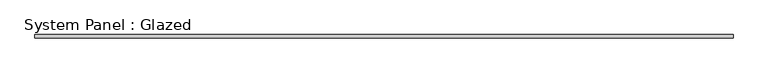
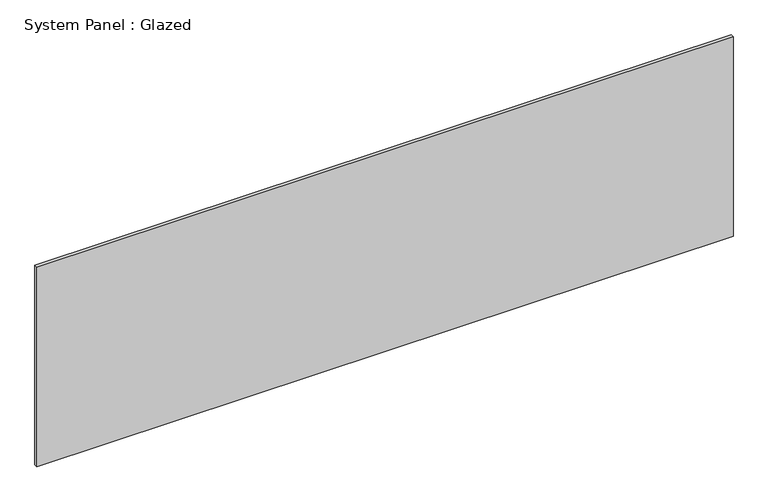
"""IFC4 building model written with IfcOpenShell, lengths in millimetres: plate geometry, System Panel : Glazed."""

from ifc_helpers import new_model, si_unit, origin, origin_with_axes, place, context, project, spatial, polyline, outline, extrude, source, transform, mapped, element, save


def system_panel_glazed_29cdcffd(model_context):
    return source(origin(), model_context, "Body", "SweptSolid", [
        extrude(outline(polyline([(2514.6, 19.05), (-2514.6, 19.05), (-2514.6, 44.45), (2514.6, 44.45), (2514.6, 19.05)])), origin_with_axes(), (0.0, 0.0, 1.0), 1524.0),
    ])


if __name__ == "__main__":
    model = new_model("IFC4")
    model_context = context("Model", 3, world=origin())
    ifc_project = project(units=[si_unit("LENGTHUNIT", "METRE", prefix="MILLI")], contexts=[model_context])
    site = spatial("IfcSite", under=ifc_project)
    building = spatial("IfcBuilding", under=site)
    placement = place(None, origin())
    system_panel_glazed_shape = system_panel_glazed_29cdcffd(model_context)
    element("IfcPlate", 1, ObjectType="System Panel : Glazed", at=placement, inside=building, context=model_context, shape_type="MappedRepresentation", body=[
        mapped(system_panel_glazed_shape, transform((0.0, 0.0, 0.0), x_axis=(1.0, 0.0, 0.0), y_axis=(0.0, 1.0, 0.0), z_axis=(0.0, 0.0, 1.0))),
    ])
    save(model, "model.ifc")

# Revit data of these elements
# Type "System Panel : Glazed"
#   Construction Type Id = "GSP4R"
#   Analytic Construction = "1/8 in Pilkington single glazing"
#   Visual Light Transmittance = 0.9
#   Solar Heat Gain Coefficient = 0.86
#   Heat Transfer Coefficient (U) = 1.18115 BTU/(h·ft²·°F)
# Element 1 (IfcPlate, "System Panel : Glazed")
#   Materials on its faces: "Glass"
# Materials
#   "Glass": class "Glass", colour RGB 0 128 192, transparency 0.75, Description = "Soda Lime Glass", Cost = 0
